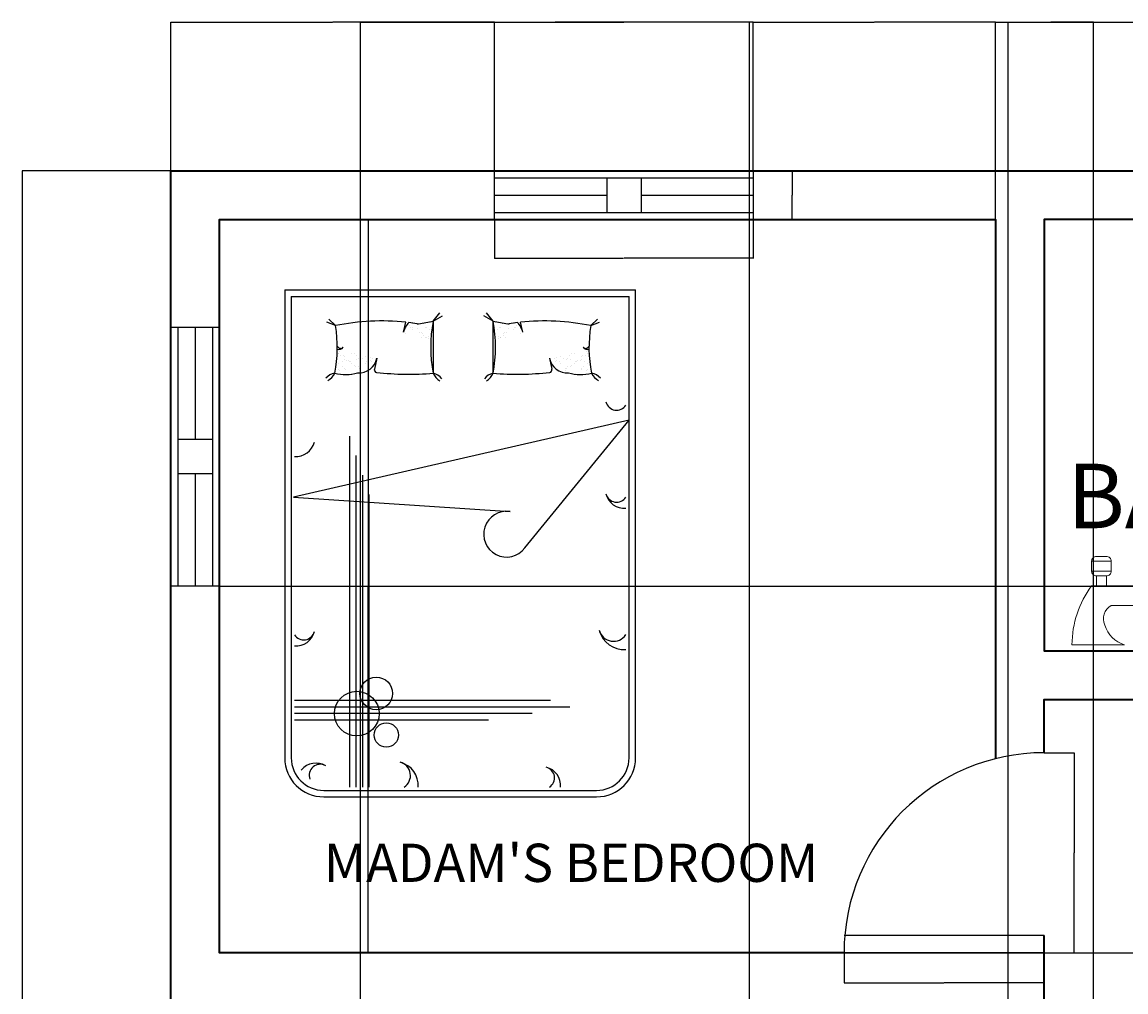
# Model space of a CAD drawing. Units: millimetres. Extents: x 19292 to 100733, y 12374 to 26974.
# Tile 19 of 24: x 42699 to 47819, y 19054 to 23551. Entities that reach past the tile are written whole.
import ezdxf

# ---------------------------------------------------------------- set-up
doc = ezdxf.new("R2010")
doc.units = ezdxf.units.MM
for name, color, linetype, lineweight in [('A-ANNO-DIMS', 2, 'Continuous', 18), ('A-AREA-IDEN', 3, 'Continuous', 25), ('A-DOOR', 4, 'Continuous', 25), ('A-FLOR-FIXT', 9, 'Continuous', 18), ('A-FURN', 8, 'Continuous', 18), ('A-GLAZ', 3, 'Continuous', 25), ('A-WALL', 7, 'Continuous', 35)]:
    doc.layers.add(name, color=color, linetype=linetype, lineweight=lineweight)
doc.layers.add('FURNITURE', color=40, linetype='Continuous')
doc.layers.add('WINDOWS', color=50, linetype='Continuous')
doc.styles.get("Standard").update_dxf_attribs({"font": 'arial.ttf'})
doc.dimstyles.get("Standard").update_dxf_attribs({"dimtxt": 0.18, "dimasz": 0.18, "dimexe": 0.18, "dimexo": 0.0625, "dimgap": 0.09, "dimtad": 0, "dimtih": 1, "dimtoh": 1, "dimdec": 4, "dimzin": 0, "dimdsep": 46, "dimtxsty": 'Standard', "dimcen": 0.09, "dimadec": 0, "dimazin": 0, "dimtfac": 1, "dimtdec": 4, "dimtofl": 0, "dimtmove": 0, "dimatfit": 3, "dimfxl": 1, "dimtolj": 1, "dimtzin": 0, "dimarcsym": 0})

# ---------------------------------------------------------------- blocks, each defined once
blk = doc.blocks.new('DBED-4FT6')
at = {"layer": 'FURNITURE'}
for p, q in [((-27, 0), (-27, -72)), ((-27, 0), (26.99999999999997, 5.68e-14)), ((27, -72.00000000000023), (26.99999999999997, 5.68e-14)), ((-26, -1), (-26, -72)), ((-26, -1), (26.00000000000003, -0.9999999999997726)), ((26, -72.00000000000023), (26.00000000000003, -0.9999999999997726)), ((-19.18306202227052, -5.485972547936796), (-20.50060919072149, -4.967335516912726)), ((-19.18306202227052, -5.485972547936967), (-20.20772305100416, -4.498686779813965)), ((-8.713720467787255, -6.492365964457349), (-8.352181760678093, -4.952469549742318)), ((-7.515425131198753, -5.088011999378352), (-7.515425131198753, -5.088011999378352)), ((-4.582631135623728, -5.081157799916695), (-4.582631135623728, -5.081157799916695)), ((-4.249112664583094, -5.02788817272858), (-4.249112664583094, -5.02788817272858)), ((-4.134652103803261, -4.817063052123046), (-3.144796483066045, -3.500606371767958)), ((-4.134652103803261, -4.817063052122875), (-2.713769052616612, -3.999588591179417)), ((5.060678666421324, -4.817063052122875), (3.639795615234675, -3.999588591179417)), ((5.060678666421324, -4.817063052123046), (4.070823045684107, -3.500606371767958)), ((5.175139227201157, -5.027888172729319), (5.175139227201157, -5.027888172729319)), ((5.50865769824179, -5.081157799916638), (5.50865769824179, -5.081157799916638)), ((8.441451693816077, -5.088011999378068), (8.441451693816077, -5.088011999378068)), ((9.639747030405317, -6.492365964457349), (9.278208323295416, -4.952469549742318)), ((20.10908858488784, -5.485972547936967), (21.13374961362223, -4.498686779813965)), ((20.10908858488858, -5.485972547936796), (21.42663575333882, -4.967335516912726)), ((-8.40590424041818, -6.637378314066779), (-8.40590424041818, -6.637378314066779)), ((-8.239079784370745, -5.562538396824265), (-8.239079784370745, -5.562538396824265)), ((-7.82267294259384, -5.507717396091834), (-7.82267294259384, -5.507717396091834)), ((-7.611546033681406, -5.809807366600068), (-7.611546033681406, -5.809807366600068)), ((-7.374544898039516, -5.845988456355428), (-7.374544898039516, -5.845988456355428)), ((-7.367969663836447, -5.22313004090148), (-7.367969663836447, -5.22313004090148)), ((-7.274189455356292, -6.024727209938816), (-7.274189455356292, -6.024727209938816)), ((-6.736049374527851, -5.364660689418656), (-6.736049374527851, -5.364660689418656)), ((-6.571710140081449, -5.952767465126385), (-6.571710140081449, -5.952767465126385)), ((-6.245189668756381, -6.559531928114552), (-6.245189668756381, -6.559531928114552)), ((-6.085661545466621, -5.279035507322305), (-6.085661545466621, -5.279035507322305)), ((-5.875720334132552, -6.590524621115605), (-5.875720334132552, -6.590524621115605)), ((-5.728264866770928, -6.725642662638733), (-5.728264866770928, -6.725642662638733)), ((-5.669254703689716, -5.224214506589873), (-5.669254703689716, -5.224214506589873)), ((-5.280472006961815, -5.819278030439932), (-5.280472006961815, -5.819278030439932)), ((-5.120232544280042, -5.805280123770785), (-5.120232544280042, -5.805280123770785)), ((-4.782875965954929, -6.020199967109533), (-4.782875965954929, -6.020199967109533)), ((5.708902528572991, -6.020199967109817), (5.708902528572991, -6.020199967109817)), ((6.046259106898105, -5.805280123771126), (6.046259106898105, -5.805280123771126)), ((6.206498569579878, -5.819278030440671), (6.206498569579878, -5.819278030440671)), ((6.595281266307779, -5.224214506589817), (6.595281266307779, -5.224214506589817)), ((6.654291429388308, -6.725642662638449), (6.654291429388308, -6.725642662638449)), ((6.801746896750614, -6.590524621115321), (6.801746896750614, -6.590524621115321)), ((7.011688108084683, -5.279035507322305), (7.011688108084683, -5.279035507322305)), ((7.171216231373705, -6.559531928115234), (7.171216231373705, -6.559531928115234)), ((7.497736702698773, -5.952767465126157), (7.497736702698773, -5.952767465126157)), ((7.662075937145914, -5.364660689418599), (7.662075937145914, -5.364660689418599)), ((8.200216017975094, -6.024727209939328), (8.200216017975094, -6.024727209939328)), ((8.293996226453771, -5.223130040901196), (8.293996226453771, -5.223130040901196)), ((8.30057146065684, -5.84598845635628), (8.30057146065684, -5.84598845635628)), ((8.537572596300208, -5.80980736660058), (8.537572596300208, -5.80980736660058)), ((8.748699505211903, -5.507717396091777), (8.748699505211903, -5.507717396091777)), ((9.165106346988807, -5.562538396824265), (9.165106346988807, -5.562538396824265)), ((9.331930803035561, -6.637378314067632), (9.331930803035561, -6.637378314067632)), ((-5.998452499838663, -7.338874652100457), (-5.998452499838663, -7.338874652100457)), ((-5.688613537228434, -7.034850473630854), (-5.688613537228434, -7.034850473630854)), ((-5.348064670777432, -7.253249470004163), (-5.348064670777432, -7.253249470004163)), ((-5.230077320474265, -7.360737045650239), (-5.230077320474265, -7.360737045650239)), ((-4.93200534301593, -7.455280086863638), (-4.93200534301593, -7.455280086863638)), ((-4.931657828999789, -7.198428469271675), (-4.931657828999789, -7.198428469271675)), ((5.857684391617851, -7.198428469271505), (5.857684391617851, -7.198428469271505)), ((5.85803190563331, -7.455280086863353), (5.85803190563331, -7.455280086863353)), ((6.156103883091589, -7.360737045650921), (6.156103883091589, -7.360737045650921)), ((6.274091233394756, -7.253249470003993), (6.274091233394756, -7.253249470003993)), ((6.614640099846496, -7.034850473631365), (6.614640099846496, -7.034850473631365)), ((6.924479062455986, -7.338874652100287), (6.924479062455986, -7.338874652100287)), ((-18.77590810264172, -9.83900715250769), (-18.77590810264172, -9.83900715250769)), ((-18.7469186025819, -9.831933062623136), (-18.7469186025819, -9.831933062623136)), ((-18.59621655837128, -9.4634697248635), (-18.59621655837128, -9.4634697248635)), ((-18.43855152431661, -10.05392699584638), (-18.43855152431661, -10.05392699584638)), ((-17.90022675242233, -10.10122688085266), (-17.90022675242233, -10.10122688085266)), ((-16.70044691192106, -9.841748322447756), (-16.70044691192106, -9.841748322447756)), ((-16.2845946132411, -9.834479909678294), (-16.2845946132411, -9.834479909678294)), ((-15.94723803491598, -10.04939975301698), (-15.94723803491598, -10.04939975301698)), ((16.87326459753331, -10.04939975301738), (16.87326459753331, -10.04939975301738)), ((17.21062117585842, -9.834479909678635), (17.21062117585842, -9.834479909678635)), ((17.62647347453912, -9.841748322448382), (17.62647347453912, -9.841748322448382)), ((18.82625331503971, -10.10122688085243), (18.82625331503971, -10.10122688085243)), ((19.36457808693467, -10.05392699584672), (19.36457808693467, -10.05392699584672)), ((19.5222431209886, -9.463469724863273), (19.5222431209886, -9.463469724863273)), ((19.67294516519922, -9.831933062623932), (19.67294516519922, -9.831933062623932)), ((19.70193466525978, -9.839007152508032), (19.70193466525978, -9.839007152508032)), ((-18.69652391609435, -11.37339207783361), (-18.69652391609435, -11.37339207783361)), ((-18.181365058572, -11.01410595179413), (-18.181365058572, -11.01410595179413)), ((-18.12980541361923, -11.84228893838752), (-18.12980541361923, -11.84228893838752)), ((-17.75277128506002, -10.23634492237579), (-17.75277128506002, -10.23634492237579)), ((-17.73180625429978, -10.63313818015905), (-17.73180625429978, -10.63313818015905)), ((-17.53097722951077, -10.92848076969778), (-17.53097722951077, -10.92848076969778)), ((-17.11457038773386, -10.87365976896535), (-17.11457038773386, -10.87365976896535)), ((-16.95651176130502, -10.9659823466007), (-16.95651176130502, -10.9659823466007)), ((-16.85297560618875, -11.06405025953836), (-16.85297560618875, -11.06405025953836)), ((-16.65005222543351, -11.38320733765818), (-16.65005222543351, -11.38320733765818)), ((-16.26052195535686, -11.60373950258992), (-16.26052195535686, -11.60373950258992)), ((-16.11306648799456, -11.73885754411304), (-16.11306648799456, -11.73885754411304)), ((-16.02794681966861, -10.73060306229217), (-16.02794681966861, -10.73060306229217)), ((-15.63849192421787, -11.83776169555784), (-15.63849192421787, -11.83776169555784)), ((-15.57109168263798, -10.55529179420631), (-15.57109168263798, -10.55529179420631)), ((-15.37755899060738, -10.64497788019582), (-15.37755899060738, -10.64497788019582)), ((-14.96115214883048, -10.59015687946339), (-14.96115214883048, -10.59015687946339)), ((-14.55597933435581, -11.35649691174245), (-14.55597933435581, -11.35649691174245)), ((-14.55161047764721, -10.26384189465318), (-14.55161047764721, -10.26384189465318)), ((-14.36166211678738, -11.05952301670902), (-14.36166211678738, -11.05952301670902)), ((-13.87452858076449, -10.44710017279021), (-13.87452858076449, -10.44710017279021)), ((-13.85562067169906, -10.9015990506424), (-13.85562067169906, -10.9015990506424)), ((-13.70816520433675, -11.03671709216553), (-13.70816520433675, -11.03671709216553)), ((-13.52461999197714, -10.56510705403116), (-13.52461999197714, -10.56510705403116)), ((-12.80860301424707, -10.50441610444505), (-13.20654336081225, -12.19935747834682)), ((13.73462957686513, -10.50441610444505), (14.13256992343031, -12.19935747834682)), ((14.45064655459447, -10.56510705403201), (14.45064655459447, -10.56510705403201)), ((14.63419176695407, -11.03671709216536), (14.63419176695407, -11.03671709216536)), ((14.78164723431638, -10.90159905064223), (14.78164723431638, -10.90159905064223)), ((14.80055514338181, -10.44710017278998), (14.80055514338181, -10.44710017278998)), ((15.28768867940545, -11.05952301670942), (15.28768867940545, -11.05952301670942)), ((15.47763704026454, -10.26384189465307), (15.47763704026454, -10.26384189465307)), ((15.48200589697319, -11.35649691174331), (15.48200589697319, -11.35649691174331)), ((15.8871787114478, -10.59015687946316), (15.8871787114478, -10.59015687946316)), ((16.30358555322471, -10.64497788019565), (16.30358555322471, -10.64497788019565)), ((16.49711824525531, -10.55529179420722), (16.49711824525531, -10.55529179420722)), ((16.56451848683594, -11.83776169555824), (16.56451848683594, -11.83776169555824)), ((16.95397338228594, -10.73060306229195), (16.95397338228594, -10.73060306229195)), ((17.03909305061188, -11.73885754411276), (17.03909305061188, -11.73885754411276)), ((17.18654851797419, -11.60373950258963), (17.18654851797419, -11.60373950258963)), ((17.57607878805157, -11.38320733765908), (17.57607878805157, -11.38320733765908)), ((17.77900216880681, -11.06405025953882), (17.77900216880681, -11.06405025953882)), ((17.8825383239224, -10.96598234660052), (17.8825383239224, -10.96598234660052)), ((18.04059695035192, -10.87365976896512), (18.04059695035192, -10.87365976896512)), ((18.45700379212883, -10.92848076969761), (18.45700379212883, -10.92848076969761)), ((18.65783281691711, -10.63313818015967), (18.65783281691711, -10.63313818015967)), ((18.6787978476774, -10.23634492237556), (18.6787978476774, -10.23634492237556)), ((19.0558319762373, -11.84228893838792), (19.0558319762373, -11.84228893838792)), ((19.10739162119006, -11.01410595179391), (19.10739162119006, -11.01410595179391)), ((19.62255047871167, -11.37339207783429), (19.62255047871167, -11.37339207783429)), ((-18.66542323901467, -12.3058799545372), (-18.66542323901467, -12.3058799545372)), ((-18.6461292296068, -12.91485109304403), (-18.6461292296068, -12.91485109304403)), ((-18.51796777165236, -12.44099799606033), (-18.51796777165236, -12.44099799606033)), ((-17.79244883529407, -12.05720878172627), (-17.79244883529407, -12.05720878172627)), ((-17.68141156781223, -12.17459719536947), (-17.68141156781223, -12.17459719536947)), ((-17.44376818388207, -12.98831991447582), (-17.44376818388207, -12.98831991447582)), ((-16.79338035482089, -12.90269473237953), (-16.79338035482089, -12.90269473237953)), ((-16.59965753894596, -12.92466635286894), (-16.59965753894596, -12.92466635286894)), ((-16.37697351304393, -12.84787373164704), (-16.37697351304393, -12.84787373164704)), ((-15.52069699614969, -12.09675080941707), (-15.52069699614969, -12.09675080941707)), ((-15.31680696423956, -12.46849496833795), (-15.31680696423956, -12.46849496833795)), ((-15.3011353458927, -12.05268153889659), (-15.3011353458927, -12.05268153889659)), ((-15.29034994497795, -12.70481702497386), (-15.29034994497795, -12.70481702497386)), ((16.21637650759675, -12.70481702497392), (16.21637650759675, -12.70481702497392)), ((16.22716190851076, -12.05268153889693), (16.22716190851076, -12.05268153889693)), ((16.24283352685688, -12.46849496833772), (16.24283352685688, -12.46849496833772)), ((16.44672355876702, -12.09675080941792), (16.44672355876702, -12.09675080941792)), ((17.303000075662, -12.8478737316471), (17.303000075662, -12.8478737316471)), ((17.52568410156328, -12.92466635286979), (17.52568410156328, -12.92466635286979)), ((17.71940691743896, -12.90269473237953), (17.71940691743896, -12.90269473237953)), ((18.36979474650013, -12.98831991447588), (18.36979474650013, -12.98831991447588)), ((18.60743813042956, -12.17459719537038), (18.60743813042956, -12.17459719537038)), ((18.71847539791213, -12.05720878172661), (18.71847539791213, -12.05720878172661)), ((19.44399433426969, -12.4409979960601), (19.44399433426969, -12.4409979960601)), ((19.57215579222412, -12.91485109304494), (19.57215579222412, -12.91485109304494)), ((19.59144980163199, -12.30587995453698), (19.59144980163199, -12.30587995453698)), ((25.99999999999997, -20.04251490499428), (-25.62857142857144, -31.89664668985566)), ((9.968437092424097, -39.68281460107684), (25.99999999999997, -20.04251490499428)), ((-16.98298633143713, -76.49999999999977), (-16.98298633143804, -22.5)), ((-15.98298633143713, -76.49999999999977), (-15.98298633143804, -25.49999999999978)), ((-14.98298633143713, -76.49999999999977), (-14.98298633143804, -28.5)), ((-25.62857142857075, -31.89664668985566), (7.69367787486118, -34.10856123257989)), ((-13.98298633143713, -76.49999999999977), (-13.98298633143804, -31.5)), ((13.92237160184822, -63.18866900046464), (-25.5, -63.18866900046464)), ((16.878192650664, -64.18866900046464), (-25.5, -64.18866900046464)), ((11.10090459947105, -65.18866900046442), (-25.5, -65.18866900046464)), ((4.383130216417612, -66.18866900046442), (-25.5, -66.18866900046464)), ((-21, -77), (21, -77.0000000000002)), ((-21, -78), (21, -78.0000000000002))]:
    blk.add_line(p, q, dxfattribs=at)
for centre, radius in [((-12.91182106300494, -62.08454274520204), 2.504372971601696), ((-15.90739414396376, -65.18866900046464), 3.437232026160017), ((-11.36543750832788, -68.48173730478015), 1.878279728701272)]:
    blk.add_circle(centre, radius, dxfattribs=at)
for centre, radius, start, end in [((-11.96490980142209, -41.81687628144138), 37.041008187906, 84.4028612645958, 101.2370836512883), ((-4.825879607851106, -7.608979000930446), 4.045013130436864, 139.9097590679286, 163.9755921234989), ((-11.52336853637479, -33.34663058587759), 28.57069839034993, 80.1409392097565, 82.7553866503384), ((-67.64177770808838, 360.6114736163754), 370.9058781068297, 279.5022474872839, 279.8588573948661), ((15.66534789619453, -8.817063052122135), 20.19999999999818, 168.5788137250011, 191.4211862750058), ((15.66534789619817, -8.817063052122649), 20.20000000000147, 168.5788137249941, 191.4211862750058), ((42751.26187429979, -8.817063056011648), 42755.39671351448, 179.9946396680611, 180.0053603319291), ((-14.73932133358011, -8.817063052122649), 20.20000000000147, 348.5788137249941, 11.42118627500586), ((-42750.33584773717, -8.817063056011648), 42755.39671351448, 359.9946396680676, 0.0053603319421324), ((-14.73932133357721, -8.817063052122135), 20.19999999999818, 348.5788137249941, 11.42118627499883), ((68.56780427070572, 360.6114736163754), 370.9058781068297, 260.141142605134, 260.4977525127162), ((12.44939509899285, -33.34663058587759), 28.57069839034993, 97.2446133496616, 99.8590607902435), ((5.751906170469169, -7.608979000930446), 4.045013130436864, 16.0244078765011, 40.09024093207139), ((12.89093636403942, -41.81687628144138), 37.041008187906, 78.76291634871168, 95.59713873540417), ((-39.10651142374138, -8.817063052122649), 20.20000000000147, 348.6069698988843, 9.491743103753544), ((-6.494365647111578, -4.409680956092984), 0.8, 260.1409392097565, 276.031827105606), ((7.420392209728902, -4.409680956092984), 0.8, 263.968172894394, 279.8590607902435), ((40.03253798635941, -8.817063052122649), 20.20000000000147, 170.5082568962464, 191.3930301011157), ((-18.63439747950781, -8.362835026573748), 0.7823789253415179, 249.4968528373028, 325.7977956221763), ((-18.4002510232591, -8.445355047199143), 0.5460297530620258, 201.8040695959829, 319.1334346759098), ((19.32627758587716, -8.445355047199143), 0.5460297530620258, 220.8665653240902, 338.1959304040171), ((19.56042404212513, -8.362835026573748), 0.7823789253415179, 214.2022043778237, 290.5031471626973), ((-15.61384730787557, -9.916934814375791), 2.86610010521538, 266.7825255240543, 348.1719149754145), ((16.53987387049363, -9.916934814375791), 2.86610010521538, 191.8280850245854, 273.2174744759457), ((-18.77582684722529, -15.36188282958866), 2.608691937302173, 101.6935339662269, 136.5635486949323), ((-21.64959486574241, -11.66451602127745), 2.608691937302173, 299.1485263283325, 334.0185410570184), ((-17.59820796861624, -5.617120538590143), 7.389908305163763, 256.6498532633935, 284.285581023734), ((-12.81713200699761, -12.29078393797522), 0.4, 166.787330358343, 262.8769841008062), ((-7.849044883706142, 31.23309670203668), 44.20648468370187, 263.4825574665681, 274.8198866450032), ((-1.728460786103994, -11.80933443470422), 2.608691937302173, 202.7242534275457, 237.5942681562781), ((-4.807664589399962, -15.33744552666542), 2.608691937302173, 40.17924578964186, 75.04926051838007), ((5.733691152018025, -15.33744552666542), 2.608691937302173, 104.9507394816199, 139.8207542103581), ((2.654487348722057, -11.80933443470422), 2.608691937302173, 302.4057318437219, 337.2757465724543), ((8.775071446323466, 31.23309670203668), 44.20648468370187, 265.1801133549968, 276.5174425334318), ((13.74315856961567, -12.29078393797522), 0.4, 277.1230158991938, 13.21266964165692), ((18.52423453123356, -5.617120538590143), 7.389908305163763, 255.7144189762659, 283.3501467366066), ((19.70185340984335, -15.36188282958866), 2.608691937302173, 43.43645130506771, 78.3064660337731), ((22.57562142836048, -11.66451602127745), 2.608691937302173, 205.9814589429815, 240.8514736716675), ((24.08149477166717, -16.81385886181465), 1.693091563593251, 194.451540940981, 326.9105817271671), ((-25.2881588087821, -22.70588367900495), 2.933920970030247, 265.8594053605621, 345.9527428336846), ((24.08149477166717, -30.96393635208892), 1.693091563593251, 194.451540940981, 326.9105817271671), ((25.28815880878119, -30.6743386403075), 2.933920970030691, 194.0472571663257, 274.140594639438), ((7.144201548013711, -37.58406550475044), 3.518672218272346, 81.0159135592615, 323.3831798465962), ((-25.28815880878119, -51.86055593582091), 2.933920970030691, 265.8594053605621, 345.9527428336743), ((-24.08149477166717, -52.15015364760233), 1.693091563593251, 213.0894182728328, 345.548459059019), ((23.60865969555653, -51.81050935983859), 2.257455418124377, 194.451540940981, 326.9105817271699), ((25.21754507837523, -51.42437907746352), 3.911894626707589, 194.0472571663257, 274.140594639438), ((-21, -72), 6, 180, 270), ((-21, -72), 5, 180, 270), ((-22.19032021997464, -75.74024097389656), 2.933920970030691, 59.04725716631266, 140.6216534048161), ((-21.541856402534, -74.6822241448225), 1.69309156359317, 59.45154094095176, 200.6983000057678), ((-9.760470192471985, -74.7268684645835), 2.116364454491481, 303.0894182728446, 75.5484590590127), ((-10.12246733219854, -76.23519851097626), 3.667401212538364, 355.8594053605848, 75.95274283367745), ((21, -72.00000000000023), 5, 270, 0), ((21, -72.00000000000023), 6, 270, 0), ((12.54583364175596, -76.28815880878142), 2.933920970030691, 355.8594053605848, 75.95274283367745), ((12.83543135353738, -75.081494771667), 1.693091563593251, 303.0894182728446, 75.5484590590127)]:
    blk.add_arc(centre, radius, start, end, dxfattribs=at)
blk = doc.blocks.new('TAP-SIDELEV')
for p, q in [((0.9999853785046433, 4.25000541523623), (1.999985378504643, 4.25000541523623)), ((1.999985378504643, 3.75000541523623), (0.9999853785046433, 3.75000541523623)), ((1.249985378504643, 3.00000541523623), (1.249985378504643, 3.50000541523623)), ((1.749985378504643, 3.50000541523623), (1.749985378504643, 3.00000541523623)), ((0.9999853785046433, 3.00000541523623), (3.840125540729427, 3.00000541523623)), ((3.527288395467852, 2.00000541523623), (1.999985378504643, 2.00000541523623)), ((4.840309954143972, 1.50000541523623), (3.840309954143972, 1.50000541523623)), ((-1.46214953567e-05, 5.415236231e-06), (0.2499853785046433, 5.415236231e-06)), ((0.2499853785046433, 5.415236231e-06), (2.675565113506539, 5.415236231e-06))]:
    blk.add_line(p, q)
for points in [[(1.249985378504643, 4.50000541523623), (1.749985378504643, 4.50000541523623)], [(0.9999853785046433, 3.75000541523623), (0.9999853785046433, 4.25000541523623)], [(1.999985378504643, 4.25000541523623), (1.999985378504643, 3.75000541523623)], [(1.749985378504643, 3.50000541523623), (1.249985378504643, 3.50000541523623)]]:
    blk.add_lwpolyline(points)
for centre, radius, start, end in [((1.242385378504675, 4.257505415236281), 0.2425917, 88.22243000000017, 181.7776), ((1.757485378504636, 4.257505415236281), 0.2425917, 358.2224, 91.77756999999983), ((1.242385378504675, 3.742405415236319), 0.2425917, 178.2223999999999, 271.7775999999998), ((1.757485378504636, 3.742405415236319), 0.2425917, 268.2224000000001, 1.777565000000075), ((5.084285378504628, -0.0280945847637639), 5.084362999999999, 143.4467, 179.6834000000001), ((3.172409954143997, 1.471305415236273), 1.668163, 0.9827694999999721, 66.40494208784), ((2.37686141733268, 1.325114461238403), 0.7729898760208992, 119.180086595352, 204.871573560288), ((3.433909954144009, 1.593605415236268), 0.4169898, 347.0191999999999, 102.9807999999998), ((3.050564044119678, 1.37500541523623), 1.425219, 195.2551000000002, 254.7449000000001)]:
    blk.add_arc(centre, radius, start, end)
blk = doc.blocks.new('WW')
at = {"layer": 'WINDOWS'}
for p, q in [((-5183.867826392408, -4940.876860268414), (-3983.867826392409, -4940.876860268414)), ((-4663.867826392415, -4940.876860268414), (-4663.867826392408, -5100.876860268415)), ((-4503.867826392416, -4940.876860268414), (-4503.867826392408, -5100.876860268415)), ((-4503.867826392416, -4940.876860268414), (-4503.867826392408, -5100.876860268415)), ((-5183.867826392408, -5020.876860268414), (-4663.867826392408, -5020.876860268415)), ((-4503.867826392416, -5020.876860268414), (-3983.867826392409, -5020.876860268414)), ((-5183.867826392408, -5100.876860268414), (-3983.867826392409, -5100.876860268414))]:
    blk.add_line(p, q, dxfattribs=at)
for points in [[(-5183.867826392408, -5133.376860268413), (-5183.867826392408, -4908.376860268414)], [(-3983.867826392409, -4908.376860268414), (-3983.867826392409, -5133.376860268413)]]:
    blk.add_lwpolyline(points, dxfattribs=at)
blk = doc.blocks.new('DOOR-900')
for p, q in [((927.6984484050844, 79.99993679812906), (-0.0003173588884238, 79.99993679812906)), ((927.6984484050844, -6.32018709439e-05), (927.6984484050844, 79.99993679812906)), ((927.6984484050844, -6.32018636679e-05), (927.6984484050844, 79.99993679813633)), ((927.6984484050844, -6.32018709439e-05), (-0.0003173588884238, -6.32018709439e-05))]:
    blk.add_line(p, q)
blk.add_arc((927.6984484050844, -6.32018709439e-05), 927.6987657639736, 90, 180)
blk = doc.blocks.new('*D26')
at = {"layer": 'A-ANNO-DIMS', "color": 0, "lineweight": -2, "transparency": 16777216}
for p, q in [((46511.29323713695, 19235.66243679812), (46511.29323713695, 19096.39012193352)), ((47438.99200290092, 19235.66243679812), (47438.99200290092, 19096.39012193352)), ((46511.47323713694, 19096.57012193352), (46973.89225849097, 19096.57012193352)), ((47438.81200290092, 19096.57012193352), (46976.39298154689, 19096.57012193352))]:
    blk.add_line(p, q, dxfattribs=at)
at = {"layer": 'A-ANNO-DIMS', "color": 0, "transparency": 16777216}
for points in [[(46511.47323713694, 19096.60012193352), (46511.47323713694, 19096.54012193352), (46511.29323713695, 19096.57012193352)], [(47438.81200290092, 19096.60012193352), (47438.81200290092, 19096.54012193352), (47438.99200290092, 19096.57012193352)]]:
    blk.add_solid(points, dxfattribs=at)
at = {"layer": 'Defpoints', "color": 0, "transparency": 16777216}
for p in [(46511.29323713695, 19235.72493679812), (47438.99200290092, 19235.72493679812), (47438.99200290092, 19096.57012193352)]:
    blk.add_point(p, dxfattribs=at)
at = {"layer": 'A-ANNO-DIMS', "color": 0, "transparency": 16777216, "insert": (46975.14262001893, 19096.57012193352), "char_height": 0.18, "attachment_point": 5}
blk.add_mtext('\\A1;DOOR 900 928 TYP.', dxfattribs=at)
blk = doc.blocks.new('*D27')
at = {"layer": 'A-ANNO-DIMS', "color": 0, "lineweight": -2, "transparency": 16777216}
for p, q in [((47439.05450290093, 20163.4237025621), (47578.32681776554, 20163.4237025621)), ((47578.14681776554, 20163.2437025621), (47578.14681776554, 19699.7562228179)), ((47578.14681776554, 19235.90493679813), (47578.14681776554, 19699.39241654232)), ((47439.05450290093, 19235.72493679813), (47578.32681776554, 19235.72493679813))]:
    blk.add_line(p, q, dxfattribs=at)
at = {"layer": 'A-ANNO-DIMS', "color": 0, "transparency": 16777216}
for points in [[(47578.11681776555, 20163.2437025621), (47578.17681776554, 20163.2437025621), (47578.14681776554, 20163.4237025621)], [(47578.11681776555, 19235.90493679813), (47578.17681776554, 19235.90493679813), (47578.14681776554, 19235.72493679813)]]:
    blk.add_solid(points, dxfattribs=at)
at = {"layer": 'Defpoints', "color": 0, "transparency": 16777216}
for p in [(47438.99200290093, 20163.4237025621), (47578.14681776554, 20163.4237025621), (47438.99200290093, 19235.72493679813)]:
    blk.add_point(p, dxfattribs=at)
at = {"layer": 'A-ANNO-DIMS', "color": 0, "transparency": 16777216, "insert": (47578.14681776554, 19699.57431968009), "char_height": 0.18, "attachment_point": 5}
blk.add_mtext('\\A1;928 TYP.', dxfattribs=at)
blk = doc.blocks.new('*D34')
at = {"layer": 'A-ANNO-DIMS', "color": 0, "lineweight": -2, "transparency": 16777216}
for p, q in [((44890.55163996643, 22635.66243679813), (44890.55163996643, 22455.54493679813)), ((46090.55163996643, 22635.66243679813), (46090.55163996643, 22455.54493679813)), ((44890.73163996643, 22455.72493679813), (45488.97878867039, 22455.72493679813)), ((46090.37163996643, 22455.72493679813), (45492.12449126248, 22455.72493679813))]:
    blk.add_line(p, q, dxfattribs=at)
at = {"layer": 'A-ANNO-DIMS', "color": 0, "transparency": 16777216}
for points in [[(44890.73163996643, 22455.75493679813), (44890.73163996643, 22455.69493679813), (44890.55163996643, 22455.72493679813)], [(46090.37163996643, 22455.75493679813), (46090.37163996643, 22455.69493679813), (46090.55163996643, 22455.72493679813)]]:
    blk.add_solid(points, dxfattribs=at)
at = {"layer": 'Defpoints', "color": 0, "transparency": 16777216}
for p in [(44890.55163996643, 22635.72493679813), (46090.55163996643, 22635.72493679813), (46090.55163996643, 22455.72493679813)]:
    blk.add_point(p, dxfattribs=at)
at = {"layer": 'A-ANNO-DIMS', "color": 0, "transparency": 16777216, "insert": (45490.55163996643, 22455.72493679813), "char_height": 0.18, "attachment_point": 5}
blk.add_mtext('\\A1;WINDOW 1200 1200 TYP.', dxfattribs=at)
blk = doc.blocks.new('*D35')
at = {"layer": 'A-ANNO-DIMS', "color": 0, "lineweight": -2, "transparency": 16777216}
for p, q in [((46090.61413996645, 22860.72493679814), (46270.73163996646, 22860.72493679814)), ((46270.55163996646, 22860.54493679813), (46270.55163996646, 22748.40683993593)), ((46270.55163996646, 22635.90493679814), (46270.55163996646, 22748.04303366035)), ((46090.61413996645, 22635.72493679813), (46270.73163996646, 22635.72493679813))]:
    blk.add_line(p, q, dxfattribs=at)
at = {"layer": 'A-ANNO-DIMS', "color": 0, "transparency": 16777216}
for points in [[(46270.52163996646, 22860.54493679813), (46270.58163996646, 22860.54493679813), (46270.55163996646, 22860.72493679814)], [(46270.52163996646, 22635.90493679814), (46270.58163996646, 22635.90493679814), (46270.55163996646, 22635.72493679813)]]:
    blk.add_solid(points, dxfattribs=at)
at = {"layer": 'Defpoints', "color": 0, "transparency": 16777216}
for p in [(46090.55163996645, 22860.72493679814), (46270.55163996646, 22860.72493679814), (46090.55163996645, 22635.72493679813)]:
    blk.add_point(p, dxfattribs=at)
at = {"layer": 'A-ANNO-DIMS', "color": 0, "transparency": 16777216, "insert": (46270.55163996646, 22748.22493679812), "char_height": 0.18, "attachment_point": 5}
blk.add_mtext('\\A1;225 TYP.', dxfattribs=at)
blk = doc.blocks.new('*D90')
at = {"layer": 'A-ANNO-DIMS', "color": 0, "lineweight": -2, "transparency": 16777216}
for p, q in [((43388.992003, 22860.787437), (43388.992003, 23550.904937)), ((43389.172003, 23550.724937), (44139.31672600204, 23550.724937)), ((44890.37163999999, 23550.724937), (44140.22691699795, 23550.724937)), ((44890.55163999999, 22860.787437), (44890.55163999999, 23550.904937))]:
    blk.add_line(p, q, dxfattribs=at)
at = {"layer": 'A-ANNO-DIMS', "color": 0, "transparency": 16777216}
for points in [[(43389.172003, 23550.754937), (43389.172003, 23550.694937), (43388.992003, 23550.724937)], [(44890.37163999999, 23550.754937), (44890.37163999999, 23550.694937), (44890.55163999999, 23550.724937)]]:
    blk.add_solid(points, dxfattribs=at)
at = {"layer": 'Defpoints', "color": 0, "transparency": 16777216}
for p in [(44890.55163999999, 23550.724937), (43388.992003, 22860.724937), (44890.55163999999, 22860.724937)]:
    blk.add_point(p, dxfattribs=at)
at = {"layer": 'A-ANNO-DIMS', "color": 0, "transparency": 16777216, "insert": (44139.7718215, 23550.724937), "char_height": 0.18, "attachment_point": 5}
blk.add_mtext('\\A1;1501.6', dxfattribs=at)
blk = doc.blocks.new('*D91')
at = {"layer": 'A-ANNO-DIMS', "color": 0, "lineweight": -2, "transparency": 16777216}
for p, q in [((44890.55163999999, 22860.787437), (44890.55163999999, 23550.904937)), ((44890.73163999999, 23550.724937), (45490.20164682128, 23550.724937)), ((46090.37164, 23550.724937), (45490.90163317871, 23550.724937)), ((46090.55163999999, 22860.787437), (46090.55163999999, 23550.904937))]:
    blk.add_line(p, q, dxfattribs=at)
at = {"layer": 'A-ANNO-DIMS', "color": 0, "transparency": 16777216}
for points in [[(44890.73163999999, 23550.754937), (44890.73163999999, 23550.694937), (44890.55163999999, 23550.724937)], [(46090.37164, 23550.754937), (46090.37164, 23550.694937), (46090.55163999999, 23550.724937)]]:
    blk.add_solid(points, dxfattribs=at)
at = {"layer": 'Defpoints', "color": 0, "transparency": 16777216}
for p in [(46090.55163999999, 23550.724937), (44890.55163999999, 22860.724937), (46090.55163999999, 22860.724937)]:
    blk.add_point(p, dxfattribs=at)
at = {"layer": 'A-ANNO-DIMS', "color": 0, "transparency": 16777216, "insert": (45490.55164, 23550.724937), "char_height": 0.18, "attachment_point": 5}
blk.add_mtext('\\A1;1200', dxfattribs=at)
blk = doc.blocks.new('*D92')
at = {"layer": 'A-ANNO-DIMS', "color": 0, "lineweight": -2, "transparency": 16777216}
for p, q in [((46090.55163999999, 22860.787437), (46090.55163999999, 23550.904937)), ((46090.73163999999, 23550.724937), (46651.81703295975, 23550.724937)), ((47213.81200299999, 23550.724937), (46652.72661004024, 23550.724937)), ((47213.992003, 22635.787437), (47213.992003, 23550.904937))]:
    blk.add_line(p, q, dxfattribs=at)
at = {"layer": 'A-ANNO-DIMS', "color": 0, "transparency": 16777216}
for points in [[(46090.73163999999, 23550.754937), (46090.73163999999, 23550.694937), (46090.55163999999, 23550.724937)], [(47213.81200299999, 23550.754937), (47213.81200299999, 23550.694937), (47213.992003, 23550.724937)]]:
    blk.add_solid(points, dxfattribs=at)
at = {"layer": 'Defpoints', "color": 0, "transparency": 16777216}
for p in [(47213.992003, 23550.724937), (46090.55163999999, 22860.724937), (47213.992003, 22635.724937)]:
    blk.add_point(p, dxfattribs=at)
at = {"layer": 'A-ANNO-DIMS', "color": 0, "transparency": 16777216, "insert": (46652.27182149999, 23550.724937), "char_height": 0.18, "attachment_point": 5}
blk.add_mtext('\\A1;1123.4', dxfattribs=at)
blk = doc.blocks.new('*D93')
at = {"layer": 'A-ANNO-DIMS', "color": 0, "lineweight": -2, "transparency": 16777216}
for p, q in [((47213.992003, 22635.787437), (47213.992003, 23550.904937)), ((47214.172003, 23550.724937), (48138.64200982128, 23550.724937)), ((49063.812003, 23550.724937), (48139.34199617871, 23550.724937)), ((49063.992003, 22860.787437), (49063.992003, 23550.904937))]:
    blk.add_line(p, q, dxfattribs=at)
at = {"layer": 'A-ANNO-DIMS', "color": 0, "transparency": 16777216}
for points in [[(47214.172003, 23550.754937), (47214.172003, 23550.694937), (47213.992003, 23550.724937)], [(49063.812003, 23550.754937), (49063.812003, 23550.694937), (49063.992003, 23550.724937)]]:
    blk.add_solid(points, dxfattribs=at)
at = {"layer": 'Defpoints', "color": 0, "transparency": 16777216}
for p in [(49063.992003, 23550.724937), (49063.992003, 22860.724937), (47213.992003, 22635.724937)]:
    blk.add_point(p, dxfattribs=at)
at = {"layer": 'A-ANNO-DIMS', "color": 0, "transparency": 16777216, "insert": (48138.99200299999, 23550.724937), "char_height": 0.18, "attachment_point": 5}
blk.add_mtext('\\A1;1850', dxfattribs=at)
blk = doc.blocks.new('*D100')
at = {"layer": 'A-ANNO-DIMS', "color": 0, "lineweight": -2, "transparency": 16777216}
for p, q in [((43388.92950300001, 22860.72493700001), (42698.81200300003, 22860.72493700001)), ((42698.99200300002, 22860.54493700001), (42698.99200300002, 18202.54073302934)), ((42698.99200300003, 13544.17260000001), (42698.99200300002, 18202.17680397067)), ((44043.61170200002, 13543.9926), (42698.81200300003, 13543.9926))]:
    blk.add_line(p, q, dxfattribs=at)
at = {"layer": 'A-ANNO-DIMS', "color": 0, "transparency": 16777216}
for points in [[(42698.96200300003, 22860.54493700001), (42699.02200300003, 22860.54493700001), (42698.99200300002, 22860.72493700001)], [(42698.96200300004, 13544.17260000001), (42699.02200300003, 13544.17260000001), (42698.99200300003, 13543.9926)]]:
    blk.add_solid(points, dxfattribs=at)
at = {"layer": 'Defpoints', "color": 0, "transparency": 16777216}
for p in [(43388.99200300001, 22860.72493700001), (42698.99200300003, 13543.9926), (44043.67420200001, 13543.9926)]:
    blk.add_point(p, dxfattribs=at)
at = {"layer": 'A-ANNO-DIMS', "color": 0, "transparency": 16777216, "insert": (42698.99200300002, 18202.35876849999), "char_height": 0.18, "attachment_point": 5}
blk.add_mtext('\\A1;9317', dxfattribs=at)
blk = doc.blocks.new('*D101')
at = {"layer": 'A-ANNO-DIMS', "color": 0, "lineweight": -2, "transparency": 16777216}
for p, q in [((43614.05450300001, 22635.72493700001), (44304.17200300003, 22635.72493700001)), ((44303.99200300002, 22635.544937), (44303.99200300002, 20935.90690152934)), ((44303.99200300002, 19235.904937), (44303.99200300002, 20935.54297247067)), ((43614.05450300001, 19235.724937), (44304.17200300003, 19235.724937))]:
    blk.add_line(p, q, dxfattribs=at)
at = {"layer": 'A-ANNO-DIMS', "color": 0, "transparency": 16777216}
for points in [[(44303.96200300003, 22635.544937), (44304.02200300003, 22635.544937), (44303.99200300002, 22635.72493700001)], [(44303.96200300003, 19235.904937), (44304.02200300003, 19235.904937), (44303.99200300002, 19235.724937)]]:
    blk.add_solid(points, dxfattribs=at)
at = {"layer": 'Defpoints', "color": 0, "transparency": 16777216}
for p in [(43613.99200300001, 22635.72493700001), (43613.99200300001, 19235.724937), (44303.99200300002, 19235.724937)]:
    blk.add_point(p, dxfattribs=at)
at = {"layer": 'A-ANNO-DIMS', "color": 0, "transparency": 16777216, "insert": (44303.99200300002, 20935.72493699999), "char_height": 0.18, "attachment_point": 5}
blk.add_mtext('\\A1;3400', dxfattribs=at)
blk = doc.blocks.new('*D102')
at = {"layer": 'A-ANNO-DIMS', "color": 0, "lineweight": -2, "transparency": 16777216}
for p, q in [((43614.05450300001, 20935.72493700001), (57530.22278900005, 20935.72493700001)), ((57530.04278900005, 20935.54493700001), (57530.04278900005, 20085.9068401378)), ((57530.04278900005, 19235.90493700001), (57530.04278900005, 20085.54303386222)), ((43614.05450300001, 19235.724937), (57530.22278900005, 19235.72493700001))]:
    blk.add_line(p, q, dxfattribs=at)
at = {"layer": 'A-ANNO-DIMS', "color": 0, "transparency": 16777216}
for points in [[(57530.01278900006, 20935.54493700001), (57530.07278900005, 20935.54493700001), (57530.04278900005, 20935.72493700001)], [(57530.01278900006, 19235.90493700001), (57530.07278900005, 19235.90493700001), (57530.04278900005, 19235.72493700001)]]:
    blk.add_solid(points, dxfattribs=at)
at = {"layer": 'Defpoints', "color": 0, "transparency": 16777216}
for p in [(43613.99200300001, 20935.72493700001), (43613.99200300001, 19235.724937), (57530.04278900005, 19235.72493700001)]:
    blk.add_point(p, dxfattribs=at)
at = {"layer": 'A-ANNO-DIMS', "color": 0, "transparency": 16777216, "insert": (57530.04278900005, 20085.72493699999), "char_height": 0.18, "attachment_point": 5}
blk.add_mtext('\\A1;1700', dxfattribs=at)
blk = doc.blocks.new('*D112')
at = {"layer": 'A-ANNO-DIMS', "color": 0, "lineweight": -2, "transparency": 16777216}
for p, q in [((43388.992003, 22860.662437), (43388.992003, 12813.8126)), ((56840.04278899999, 15985.662601), (56840.04278899999, 12813.8126)), ((43389.172003, 12813.9926), (50114.11454470395, 12813.9926)), ((56839.86278899999, 12813.9926), (50114.92024729603, 12813.9926))]:
    blk.add_line(p, q, dxfattribs=at)
at = {"layer": 'A-ANNO-DIMS', "color": 0, "transparency": 16777216}
for points in [[(43389.172003, 12814.0226), (43389.172003, 12813.9626), (43388.992003, 12813.9926)], [(56839.86278899999, 12814.0226), (56839.86278899999, 12813.9626), (56840.04278899999, 12813.9926)]]:
    blk.add_solid(points, dxfattribs=at)
at = {"layer": 'Defpoints', "color": 0, "transparency": 16777216}
for p in [(43388.992003, 22860.724937), (56840.04278899999, 15985.725101), (56840.04278899999, 12813.9926)]:
    blk.add_point(p, dxfattribs=at)
at = {"layer": 'A-ANNO-DIMS', "color": 0, "transparency": 16777216, "insert": (50114.517396, 12813.9926), "char_height": 0.18, "attachment_point": 5}
blk.add_mtext('\\A1;13451', dxfattribs=at)
blk = doc.blocks.new('*D114')
at = {"layer": 'A-ANNO-DIMS', "color": 0, "lineweight": -2, "transparency": 16777216}
for p, q in [((44267.980129, 13769.0551), (44267.980129, 23550.904937)), ((44268.160129, 23550.724937), (45170.14306305662, 23550.724937)), ((46072.82794799999, 23550.724937), (45170.84501394339, 23550.724937)), ((46073.007948, 13769.0551), (46073.007948, 23550.904937))]:
    blk.add_line(p, q, dxfattribs=at)
at = {"layer": 'A-ANNO-DIMS', "color": 0, "transparency": 16777216}
for points in [[(44268.160129, 23550.754937), (44268.160129, 23550.694937), (44267.980129, 23550.724937)], [(46072.82794799999, 23550.754937), (46072.82794799999, 23550.694937), (46073.007948, 23550.724937)]]:
    blk.add_solid(points, dxfattribs=at)
at = {"layer": 'Defpoints', "color": 0, "transparency": 16777216}
for p in [(46073.007948, 23550.724937), (44267.980129, 13768.9926), (46073.007948, 13768.9926)]:
    blk.add_point(p, dxfattribs=at)
at = {"layer": 'A-ANNO-DIMS', "color": 0, "transparency": 16777216, "insert": (45170.4940385, 23550.724937), "char_height": 0.18, "attachment_point": 5}
blk.add_mtext('\\A1;1805', dxfattribs=at)
blk = doc.blocks.new('*D115')
at = {"layer": 'A-ANNO-DIMS', "color": 0, "lineweight": -2, "transparency": 16777216}
for p, q in [((47273.00794799999, 13769.0551), (47273.00794799999, 23550.904937)), ((47273.187948, 23550.724937), (47470.2045773813, 23550.724937)), ((47667.800129, 23550.724937), (47470.78349961869, 23550.724937)), ((47667.980129, 13769.0551), (47667.980129, 23550.904937))]:
    blk.add_line(p, q, dxfattribs=at)
at = {"layer": 'A-ANNO-DIMS', "color": 0, "transparency": 16777216}
for points in [[(47273.187948, 23550.754937), (47273.187948, 23550.694937), (47273.00794799999, 23550.724937)], [(47667.800129, 23550.754937), (47667.800129, 23550.694937), (47667.980129, 23550.724937)]]:
    blk.add_solid(points, dxfattribs=at)
at = {"layer": 'Defpoints', "color": 0, "transparency": 16777216}
for p in [(47667.980129, 23550.724937), (47273.00794799999, 13768.9926), (47667.980129, 13768.9926)]:
    blk.add_point(p, dxfattribs=at)
at = {"layer": 'A-ANNO-DIMS', "color": 0, "transparency": 16777216, "insert": (47470.4940385, 23550.724937), "char_height": 0.18, "attachment_point": 5}
blk.add_mtext('\\A1;395', dxfattribs=at)

msp = doc.modelspace()

# ---------------------------------------------------------------- linework, layer by layer
at = {"layer": 'A-WALL'}
for points in [[(43388.99200290092, 22860.72493679813), (49063.99200290092, 22860.72493679813), (49063.99200290092, 22460.72493679813), (56838.99200290092, 22460.72493679813), (56840.04278867613, 15985.72510139728), (54414.5194911604, 15985.331478935), (54414.5194911604, 14906.40305703235), (52089.65806670906, 14906.40305703235), (52089.65806670906, 13543.99260027244), (44043.67420168258, 13543.99260027244), (44026.77842884958, 19012.69540309651), (43388.99200290092, 19010.72493679813), (43388.99200290092, 22860.72493679813)], [(46511.29323713695, 19235.72493679813), (43613.99200290092, 19235.72493679813), (43613.99200290092, 22635.72493679813), (47213.99200290092, 22635.72493679813), (47213.99200290092, 20135.72493679813)], [(48838.99200290092, 20635.72493679813), (48838.99200290092, 22635.72493679813), (47438.99200290092, 22635.72493679813), (47438.99200290092, 20635.72493679813), (48138.99200290092, 20635.72493679813)], [(47438.99200290092, 20163.4237025621), (47438.99200290092, 20410.72493679813), (48103.71994440829, 20410.72493679813)], [(46492.98012915374, 18622.46175558771), (46492.98012915374, 18993.99260027244), (47438.99200290092, 18993.99260027244), (47438.99200290092, 19315.72493679813)]]:
    msp.add_lwpolyline(points, dxfattribs=at)

# ---------------------------------------------------------------- block references
at = {"layer": 'A-DOOR'}
msp.add_blockref('DOOR-900', (46511.29355449584, 19235.72499999999), dxfattribs=at)
at = {"layer": 'A-FLOR-FIXT', "xscale": 91.03318940714036, "yscale": 91.03318940714036, "zscale": 91.03318940714036}
msp.add_blockref('TAP-SIDELEV', (47568.66924331107, 20664.11646602613), dxfattribs=at)
at = {"layer": 'A-FURN', "xscale": 30.13269765108242, "yscale": 30.13269765108242, "zscale": 30.13269765108242}
msp.add_blockref('DBED-4FT6', (44730.64312069601, 22309.03809122464), dxfattribs=at)
at = {"layer": 'A-GLAZ'}
msp.add_blockref('WW', (50074.41946635884, 27769.10179706654), dxfattribs=at)
at = {"layer": 'A-GLAZ', "rotation": 270}
msp.add_blockref('WW', (48522.36886316934, 16951.85711040572), dxfattribs=at)

# ---------------------------------------------------------------- texts
at = {"layer": 'A-AREA-IDEN'}
for s, height, p in [('BATH', 299.1707480039913, (47545.65666395047, 21204.25078567758)), ("MADAM'S BEDROOM", 177.1874936163484, (44097.85647002328, 19564.32757063303))]:
    msp.add_text(s, height=height, dxfattribs=at).set_placement(p)

# ---------------------------------------------------------------- dimensions: what is measured, and where the dimension line sits
at = {"layer": 'A-ANNO-DIMS'}
for base, p1, p2, override, picture, middle in [((44890.55163999999, 23550.724937), (43388.992003, 22860.724937), (44890.55163999999, 22860.724937), {"dimdec": 1, "dimlfac": 1, "dimrnd": 0, "dimzin": 0, "dimdsep": 46, "dimlunit": 2}, '*D90', (44139.7718215, 23550.724937)), ((46073.007948, 23550.724937), (44267.980129, 13768.9926), (46073.007948, 13768.9926), {"dimdec": 0, "dimlfac": 1, "dimrnd": 0, "dimzin": 0, "dimdsep": 46, "dimlunit": 2}, '*D114', (45170.4940385, 23550.724937)), ((46090.55163999999, 23550.724937), (44890.55163999999, 22860.724937), (46090.55163999999, 22860.724937), {"dimdec": 0, "dimlfac": 1, "dimrnd": 0, "dimzin": 0, "dimdsep": 46, "dimlunit": 2}, '*D91', (45490.55164, 23550.724937)), ((47213.992003, 23550.724937), (46090.55163999999, 22860.724937), (47213.992003, 22635.724937), {"dimdec": 1, "dimlfac": 1, "dimrnd": 0, "dimzin": 0, "dimdsep": 46, "dimlunit": 2}, '*D92', (46652.27182149999, 23550.724937)), ((49063.992003, 23550.724937), (47213.992003, 22635.724937), (49063.992003, 22860.724937), {"dimdec": 0, "dimlfac": 1, "dimrnd": 0, "dimzin": 0, "dimdsep": 46, "dimlunit": 2}, '*D93', (48138.99200299999, 23550.724937)), ((47667.980129, 23550.724937), (47273.00794799999, 13768.9926), (47667.980129, 13768.9926), {"dimdec": 0, "dimlfac": 1, "dimrnd": 0, "dimzin": 0, "dimdsep": 46, "dimlunit": 2}, '*D115', (47470.4940385, 23550.724937)), ((56840.04278899999, 12813.9926), (43388.992003, 22860.724937), (56840.04278899999, 15985.725101), {"dimdec": 0, "dimlfac": 1, "dimrnd": 0, "dimzin": 0, "dimdsep": 46, "dimlunit": 2}, '*D112', (50114.517396, 12813.9926))]:
    dim = msp.add_linear_dim(base=base, p1=p1, p2=p2, dimstyle='Standard', override=override, dxfattribs=at)
    dim.commit()
    dim.dimension.update_dxf_attribs({"geometry": picture, "text_midpoint": middle})
for base, p1, p2, angle, picture, middle in [((42698.99200300003, 13543.9926), (43388.992003, 22860.724937), (44043.674202, 13543.9926), 90, '*D100', (42698.99200300002, 18202.35876849999)), ((44303.99200300002, 19235.724937), (43613.992003, 22635.724937), (43613.992003, 19235.724937), 270, '*D101', (44303.99200300002, 20935.72493699999)), ((57530.04278900005, 19235.72493700001), (43613.992003, 20935.724937), (43613.992003, 19235.724937), 90, '*D102', (57530.04278900005, 20085.72493699999))]:
    dim = msp.add_linear_dim(base=base, p1=p1, p2=p2, angle=angle, dimstyle='Standard', override={"dimdec": 0, "dimlfac": 1, "dimrnd": 0, "dimzin": 0, "dimdsep": 46, "dimlunit": 2}, dxfattribs=at)
    dim.commit()
    dim.dimension.update_dxf_attribs({"geometry": picture, "text_midpoint": middle})
for base, p1, p2, picture, middle in [((46270.55163996646, 22860.72493679814), (46090.55163996643, 22635.72493679813), (46090.55163996643, 22860.72493679813), '*D35', (46270.55163996646, 22748.22493679812)), ((47578.14681776554, 20163.4237025621), (47438.99200290092, 19235.72493679812), (47438.99200290092, 20163.42370256209), '*D27', (47578.14681776554, 19699.57431968009))]:
    dim = msp.add_linear_dim(base=base, p1=p1, p2=p2, angle=90, text='<> TYP.', dimstyle='Standard', override={"dimdec": 0, "dimrnd": 0, "dimzin": 0, "dimlunit": 2}, dxfattribs=at)
    dim.commit()
    dim.dimension.update_dxf_attribs({"geometry": picture, "text_midpoint": middle})
for base, p1, p2, text, picture, middle in [((46090.55163996643, 22455.72493679813), (44890.55163996643, 22635.72493679813), (46090.55163996643, 22635.72493679813), 'WINDOW 1200 <> TYP.', '*D34', (45490.55163996643, 22455.72493679813)), ((47438.99200290092, 19096.57012193352), (46511.29323713695, 19235.72493679812), (47438.99200290092, 19235.72493679812), 'DOOR 900 <> TYP.', '*D26', (46975.14262001893, 19096.57012193352))]:
    dim = msp.add_linear_dim(base=base, p1=p1, p2=p2, text=text, dimstyle='Standard', override={"dimdec": 0, "dimrnd": 0, "dimzin": 0, "dimlunit": 2}, dxfattribs=at)
    dim.commit()
    dim.dimension.update_dxf_attribs({"geometry": picture, "text_midpoint": middle})

doc.saveas('drawing.dxf')
